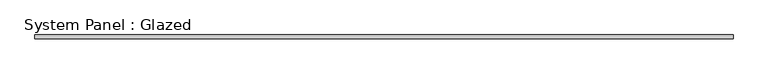
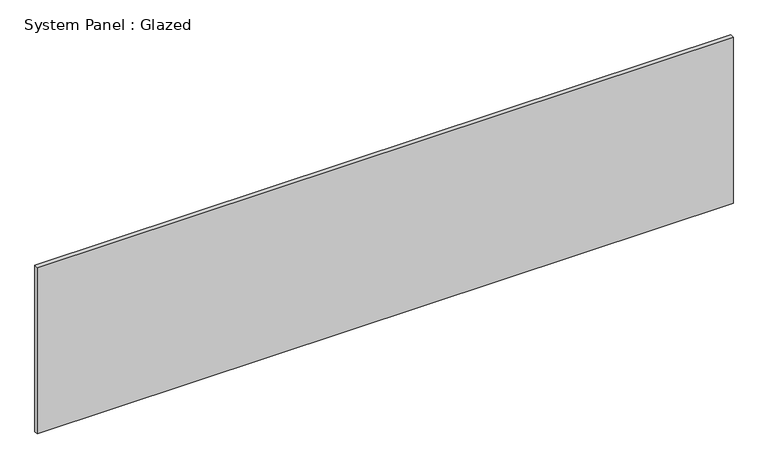
"""IFC4 building model written with IfcOpenShell, lengths in millimetres: plate geometry, System Panel : Glazed."""

from ifc_helpers import new_model, si_unit, origin, origin_with_axes, place, context, project, spatial, polyline, outline, extrude, source, transform, mapped, element, save


def system_panel_glazed_6b3781c5(model_context):
    return source(origin(), model_context, "Body", "SweptSolid", [
        extrude(outline(polyline([(2288.0184088, 19.05), (-2288.0184088, 19.05), (-2288.0184088, 44.45), (2288.0184088, 44.45), (2288.0184088, 19.05)])), origin_with_axes(), (0.0, 0.0, 1.0), 1155.7),
    ])


if __name__ == "__main__":
    model = new_model("IFC4")
    model_context = context("Model", 3, world=origin())
    ifc_project = project(units=[si_unit("LENGTHUNIT", "METRE", prefix="MILLI")], contexts=[model_context])
    site = spatial("IfcSite", under=ifc_project)
    building = spatial("IfcBuilding", under=site)
    placement = place(None, origin())
    system_panel_glazed_shape = system_panel_glazed_6b3781c5(model_context)
    element("IfcPlate", 1, ObjectType="System Panel : Glazed", at=placement, inside=building, context=model_context, shape_type="MappedRepresentation", body=[
        mapped(system_panel_glazed_shape, transform((0.0, 0.0, 0.0), x_axis=(1.0, 0.0, 0.0), y_axis=(0.0, 1.0, 0.0), z_axis=(0.0, 0.0, 1.0))),
    ])
    save(model, "model.ifc")

# Revit data of these elements
# Type "System Panel : Glazed"
#   Construction Type Id = "GSP4R"
#   Analytic Construction = "1/8 in Pilkington single glazing"
#   Visual Light Transmittance = 0.9
#   Solar Heat Gain Coefficient = 0.86
#   Heat Transfer Coefficient (U) = 1.18115 BTU/(h·ft²·°F)
# Element 1 (IfcPlate, "System Panel : Glazed")
#   Materials on its faces: "Glass"
# Materials
#   "Glass": class "Glass", colour RGB 0 128 192, transparency 0.75, Description = "Soda Lime Glass", Cost = 0
